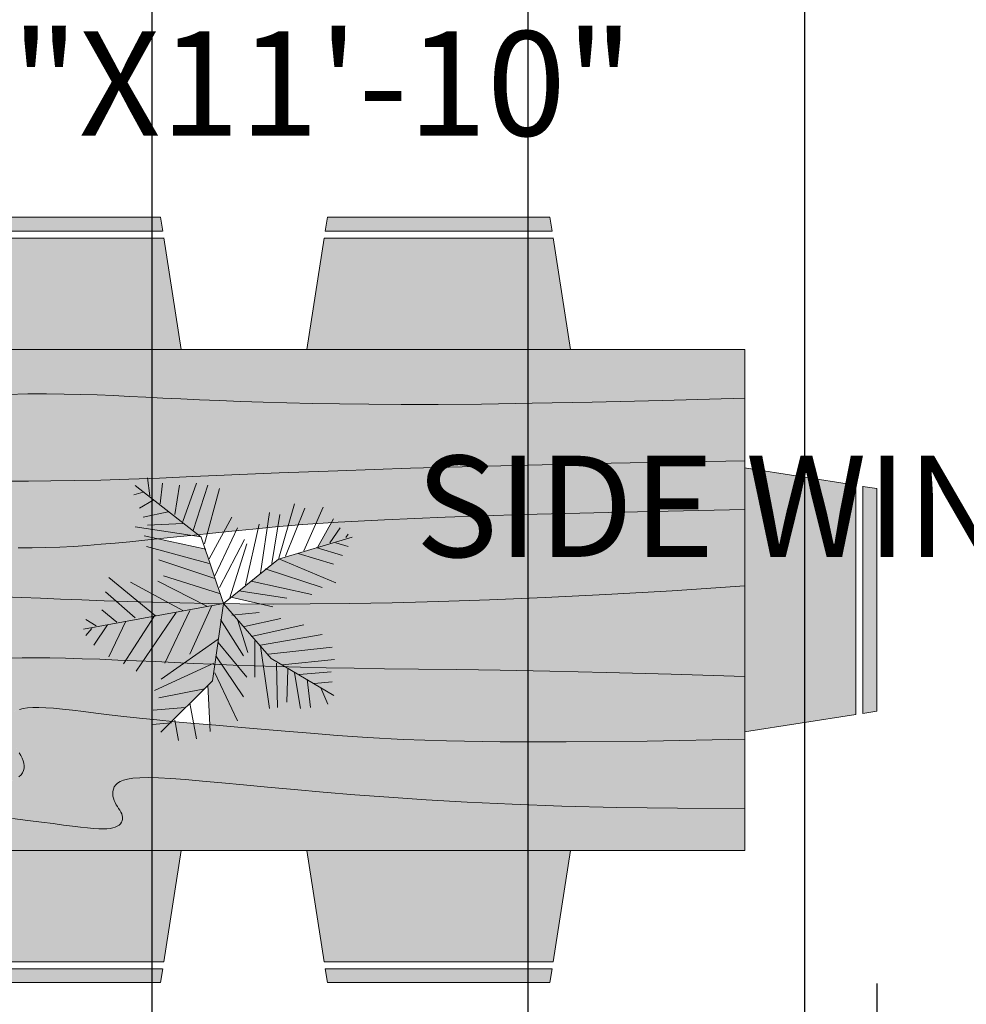
# Model space of a CAD drawing. Units: inches. Extents: x 2974 to 3443, y 2405 to 2963.
# Tile 8 of 13: x 3276 to 3341, y 2643 to 2711. Entities that reach past the tile are written whole.
import ezdxf

# ---------------------------------------------------------------- set-up
doc = ezdxf.new("R2010")
doc.units = ezdxf.units.IN
doc.header["$MEASUREMENT"] = 0
doc.layers.get('0').update_dxf_attribs({"color": 251})
for name, color, linetype, lineweight in [('A-ANNO-DIMS', 2, 'Continuous', 18), ('A-AREA-IDEN', 250, 'Continuous', 25), ('furniture', 32, 'Continuous', 18), ('greenary', 106, 'Continuous', 13)]:
    doc.layers.add(name, color=color, linetype=linetype, lineweight=lineweight)
doc.layers.add('A-FURN-PATT', color=254, linetype='Continuous', lineweight=13, true_color=0xfeeab9)
doc.styles.get("Standard").update_dxf_attribs({"font": 'arial.ttf'})
doc.dimstyles.get("Standard").update_dxf_attribs({"dimtxt": 7, "dimasz": 0.18, "dimexe": 0.18, "dimexo": 0.0625, "dimgap": 0.09, "dimtad": 0, "dimtih": 1, "dimtoh": 1, "dimzin": 0, "dimdsep": 46, "dimlunit": 3, "dimtxsty": 'Standard', "dimcen": 0.09, "dimadec": 0, "dimazin": 0, "dimtfac": 1, "dimtofl": 0, "dimtmove": 0, "dimatfit": 3, "dimfxl": 1, "dimtolj": 1, "dimtzin": 0, "dimarcsym": 0})

# ---------------------------------------------------------------- blocks, each defined once
blk = doc.blocks.new('Dining Set - 36 x 72 in.')
for p, q in [((-22, 27.5), (-22.1562, 26.50042)), ((-22, 27.5), (-6, 27.5)), ((-5.8437, 26.49966), (-6, 27.5)), ((6, 27.5), (5.8438, 26.50042)), ((6, 27.5), (22, 27.5)), ((-5.8416, 26.5), (-22.1534, 26.5)), ((22.1584, 26.5), (5.8466, 26.5)), ((-22.2343, 26.00059), (-23.4847, 17.99762)), ((-22.2304, 26), (-5.7608, 26)), ((-4.5152, 17.99762), (-5.7655, 25.99926)), ((5.7657, 26.00059), (4.5153, 17.99762)), ((5.7696, 26), (22.2392, 26)), ((36, 18), (-36, 18)), ((-36, 18), (-36, -18)), ((-44.0006, 8.23428), (-35.9976, 9.48474)), ((-45.5, 8), (-44.5004, 8.15617)), ((-45.5, 8), (-45.5, -8)), ((-44.5, -8.15843), (-44.5, 8.15338)), ((-44, 8.23041), (-44, -8.23915)), ((-44.4997, -8.15631), (-45.5, -8)), ((-35.9976, -9.48476), (-43.9993, -8.2345)), ((-36, -18), (36, -18)), ((-22.2343, -26.0006), (-23.4847, -17.99762)), ((-4.5152, -17.99762), (-5.7655, -25.99928)), ((5.7657, -26.0006), (4.5153, -17.99762)), ((-22.2304, -26), (-5.7608, -26)), ((5.7696, -26), (22.2392, -26)), ((-22, -27.5), (-22.1562, -26.50044)), ((-5.8416, -26.5), (-22.1534, -26.5)), ((-5.8437, -26.49967), (-6, -27.5)), ((6, -27.5), (5.8438, -26.50044)), ((22.1584, -26.5), (5.8466, -26.5)), ((-22, -27.5), (-6, -27.5)), ((6, -27.5), (22, -27.5))]:
    blk.add_line(p, q)
for points in [[(-36, 15), (-31.1772, 14.97754), (-26.8079, 14.91406), (-22.8538, 14.81543), (-19.276, 14.6875), (-16.0362, 14.53613), (-13.0957, 14.36718), (-10.4159, 14.18652), (-7.9583, 14), (-5.6904, 13.81315), (-3.6035, 13.63021), (-1.6954, 13.45508), (0.0365, 13.29166), (1.5945, 13.14388), (2.9811, 13.01562), (4.1988, 12.9108), (5.25, 12.83333), (6.1393, 12.78613), (6.8802, 12.76823), (7.4883, 12.77767), (7.9792, 12.8125), (8.3685, 12.87077), (8.6719, 12.95052), (8.9049, 13.0498), (9.0833, 13.16666), (9.2205, 13.29899), (9.3216, 13.44401), (9.3895, 13.59879), (9.4271, 13.76041), (9.4373, 13.92594), (9.4232, 14.09245), (9.3875, 14.257), (9.3333, 14.41666), (9.2638, 14.56917), (9.1836, 14.71484), (9.0975, 14.85465), (9.0104, 14.98958), (8.9272, 15.1206), (8.8529, 15.2487), (8.7922, 15.37483), (8.75, 15.5), (8.7305, 15.62467), (8.7344, 15.74739), (8.7617, 15.86621), (8.8125, 15.97916), (8.8867, 16.08431), (8.9844, 16.17968), (9.1055, 16.26334), (9.25, 16.33333), (9.4189, 16.38802), (9.6172, 16.42708), (9.8506, 16.45052), (10.125, 16.45833), (10.4463, 16.45052), (10.8203, 16.42708), (11.2529, 16.38802), (11.75, 16.33333), (12.3184, 16.26318), (12.9694, 16.17838), (13.7151, 16.07991), (14.5677, 15.96875), (15.5395, 15.84586), (16.6426, 15.71224)], [(-36, 10), (-28.9766, 10.14274), (-23.1725, 10.20442), (-18.4241, 10.19775), (-14.5677, 10.13541), (-11.4399, 10.03011), (-8.877, 9.89453), (-6.7154, 9.74137), (-4.7917, 9.58333), (-2.9698, 9.43082), (-1.2246, 9.28515), (0.4415, 9.14534), (2.026, 9.01041), (3.5266, 8.87939), (4.9408, 8.7513), (6.266, 8.62516), (7.5, 8.5), (8.6411, 8.37549), (9.6914, 8.2539), (10.6538, 8.13818), (11.5312, 8.03125), (12.3267, 7.93603), (13.043, 7.85547), (13.6831, 7.79248), (14.25, 7.75), (14.7471, 7.7303), (15.1797, 7.73307), (15.5537, 7.75732), (15.875, 7.80208), (16.1494, 7.86637)], [(16.1667, 11), (16.05, 11.18733), (15.9518, 11.3737), (15.8752, 11.5581), (15.8229, 11.73958), (15.798, 11.91715), (15.8034, 12.08984), (15.842, 12.25667), (15.9167, 12.41666), (16.0295, 12.56836), (16.1784, 12.70833)], [(-36, 5.5), (-30.7157, 5.3348), (-26.069, 5.20963), (-21.9946, 5.11767), (-18.4271, 5.05208), (-15.3009, 5.00602), (-12.5508, 4.97265), (-10.1112, 4.94515), (-7.9167, 4.91666), (-5.909, 4.88167), (-4.0586, 4.83984), (-2.3429, 4.79215), (-0.7396, 4.73958), (0.7739, 4.6831), (2.22, 4.6237), (3.6213, 4.56233), (5, 4.5), (6.373, 4.43782), (7.7344, 4.3776), (9.0723, 4.32129), (10.375, 4.27083), (11.6309, 4.22819), (12.8281, 4.19531), (13.9551, 4.17415), (15, 4.16666), (15.954, 4.17448), (16.819, 4.19791)], [(-36, -1), (-30.7915, -0.6591), (-26.0195, -0.38216), (-21.6519, -0.16284), (-17.6563, 0.00521), (-14.0005, 0.12833), (-10.6523, 0.21289), (-7.5796, 0.26522), (-4.75, 0.29166), (-2.134, 0.29793), (0.2878, 0.28711), (2.5317, 0.26163), (4.6146, 0.22396), (6.5529, 0.17651), (8.3633, 0.12174), (10.0623, 0.06209), (11.6667, 0), (13.1899, -0.06201), (14.6341, -0.1211), (15.9982, -0.17432), (17.2813, -0.21875)], [(-36, -6.5), (-27.1843, -6.31267), (-20.084, -6.1263), (-14.469, -5.9419), (-10.1094, -5.76042), (-6.7752, -5.58285), (-4.2363, -5.41016), (-2.2629, -5.24333), (-0.625, -5.08334), (0.8708, -4.93099), (2.2715, -4.78646), (3.5872, -4.64974), (4.8281, -4.52084), (6.0046, -4.39974), (7.127, -4.28646), (8.2053, -4.18099), (9.25, -4.08334), (10.2705, -3.99382), (11.2734, -3.91407), (12.2647, -3.84603), (13.25, -3.79167), (14.2354, -3.75293), (15.2266, -3.73177), (16.2295, -3.73015)], [(-36, -10), (-26.4022, -9.81299), (-18.4675, -9.62891), (-11.9839, -9.45069), (-6.7396, -9.28125), (-2.5226, -9.12354), (0.8789, -8.98047), (3.6769, -8.85498), (6.0833, -8.75), (8.2767, -8.66765), (10.3021, -8.60677), (12.1712, -8.56543), (13.8958, -8.54167), (15.4876, -8.53353), (16.9583, -8.53907)], [(-36, -14.5), (-30.0881, -14.33513), (-25.0332, -14.21224), (-20.7312, -14.12647), (-17.0781, -14.07292), (-13.97, -14.04671), (-11.3027, -14.04297), (-8.9724, -14.05681), (-6.875, -14.08334), (-4.9224, -14.11833), (-3.0905, -14.16016), (-1.3709, -14.20785), (0.2448, -14.26042), (1.7647, -14.3169), (3.1973, -14.3763), (4.5507, -14.43767), (5.8333, -14.5), (7.0554, -14.5621), (8.235, -14.62175), (9.3922, -14.67652), (10.5469, -14.72396), (11.7192, -14.76164), (12.929, -14.78711), (14.1965, -14.79794), (15.5417, -14.79167), (16.9933, -14.76424)]]:
    blk.add_lwpolyline(points)
blk = doc.blocks.new('dining area')
at = {"layer": 'furniture', "xscale": 0.6659924291999282, "yscale": 0.6659924291999282, "zscale": 0.6659924291999282, "rotation": 90}
blk.add_blockref('Dining Set - 36 x 72 in.', (-0.439, 20.507), dxfattribs=at)
blk = doc.blocks.new('*U13')
for p, q in [((0, 0), (-10.5, 57)), ((-8.737, 47.138), (-17.069, 52.711)), ((-10.186, 53.64), (-13.084, 55.962)), ((-9.099, 51.782), (-6.563, 55.962)), ((-7.65, 43.423), (-2.578, 49.46)), ((-7.288, 39.707), (-21.778, 46.673)), ((-5.839, 35.992), (4.667, 48.067)), ((-5.114, 27.632), (10.463, 46.673)), ((-5.114, 28.097), (-24.676, 40.636)), ((-2.941, 16.486), (8.652, 37.85)), ((44.153, 36.456), (45.239, 32.741)), ((-3.665, 19.273), (-27.574, 35.527)), ((22.055, 7.198), (27.489, 32.277)), ((27, 9), (48, 36)), ((27.127, 9.056), (31.112, 35.992)), ((35.096, 32.741), (37.27, 22.524)), ((38.719, 34.134), (41.979, 28.561)), ((-48.585, 21.131), (-49.309, 29.026)), ((-43.513, 28.561), (-42.427, 15.558)), ((-35.544, 28.097), (-24.314, 3.947)), ((16.259, 5.805), (23.142, 31.348)), ((31.836, 30.883), (32.561, 16.486)), ((43.791, 29.954), (51.036, 30.883)), ((-31.5, 4.5), (-52.5, 25.5)), ((-38.442, 26.239), (-34.819, 7.663)), ((-14.533, 2.09), (-30.834, 25.31)), ((-1.129, 6.734), (9.014, 26.704)), ((3.942, 1.625), (11.187, 24.381)), ((10.101, 3.483), (17.708, 26.239)), ((40.53, 25.775), (48.862, 24.846)), ((-24.314, 23.917), (-2.941, 13.7)), ((-47.498, 19.737), (-55.83, 18.344)), ((33.285, 16.486), (48.862, 10.913)), ((36.183, 19.737), (48.137, 17.88)), ((-40.615, 13.7), (-55.105, 10.913)), ((-20.691, 13.7), (-1.129, 4.876)), ((29.662, 12.307), (48.137, 6.269)), ((0, 0), (27, 9)), ((-33.37, 6.269), (-52.207, 5.34)), ((0, 0), (-31.5, 4.5)), ((18.07, 5.805), (35.096, -3.483)), ((24.229, 7.663), (46.688, 1.625)), ((-28.299, 3.483), (-47.86, -5.805)), ((-21.416, 3.018), (-38.079, -8.128)), ((-15.982, 2.09), (-30.11, -9.521)), ((0, 0), (-22.5, -19.5)), ((-6.563, 1.161), (-21.416, -8.128)), ((0, 0), (18, -22.5)), ((6.478, 1.625), (26.04, -8.592)), ((11.187, 3.483), (30.749, -5.805)), ((-4.752, -3.483), (-3.665, -14.629)), ((2.493, -3.019), (-1.491, -20.202)), ((1.769, -2.555), (24.229, -9.521)), ((-6.563, -5.805), (-19.967, -9.985)), ((5.029, -6.27), (2.131, -25.775)), ((-13.446, -11.378), (-8.737, -32.741)), ((-9.461, -8.592), (-6.201, -23.453)), ((9.014, -11.378), (3.58, -35.992)), ((7.565, -9.056), (32.198, -14.629)), ((-17.431, -15.094), (-42.789, -18.809)), ((-15.257, -12.772), (-30.11, -12.772)), ((-17.069, -15.094), (-12.721, -40.172)), ((12.274, -15.094), (36.907, -18.809)), ((-22.5, -19.5), (-37.5, -45)), ((-20.691, -18.345), (-17.793, -44.352)), ((14.085, -16.951), (6.478, -40.172)), ((16.259, -19.738), (36.183, -22.989)), ((-24.314, -21.596), (-42.427, -22.06)), ((-25.038, -23.918), (-22.865, -45.281)), ((18.07, -22.524), (8.289, -45.745)), ((18, -22.5), (27, -52.5)), ((18.433, -22.524), (40.53, -29.026)), ((-26.849, -26.24), (-40.253, -25.775)), ((19.157, -25.311), (38.719, -33.206)), ((-28.299, -29.026), (-42.789, -31.348)), ((-29.023, -30.884), (-27.936, -43.887)), ((20.244, -30.419), (15.897, -44.816)), ((-30.834, -34.135), (-42.427, -35.528)), ((21.331, -32.741), (39.081, -40.636)), ((-34.457, -39.708), (-40.978, -42.494)), ((-32.646, -36.921), (-31.921, -44.352)), ((22.78, -37.85), (19.519, -48.532)), ((22.78, -38.314), (34.372, -44.816)), ((24.591, -43.423), (30.749, -47.603)), ((24.591, -45.745), (23.142, -50.854)), ((26.764, -49.925), (28.213, -50.854))]:
    blk.add_line(p, q)
blk = doc.blocks.new('*D31')
at = {"layer": 'A-ANNO-DIMS', "color": 0, "lineweight": -2, "transparency": 16777216}
for p, q in [((3375.263, 2710.653), (3365.052, 2710.653)), ((3365.232, 2710.473), (3365.232, 2680.719)), ((3365.232, 2643.541), (3365.232, 2673.295)), ((3375.263, 2643.361), (3365.052, 2643.361))]:
    blk.add_line(p, q, dxfattribs=at)
at = {"layer": 'A-ANNO-DIMS', "color": 0, "transparency": 16777216}
for points in [[(3365.202, 2710.473), (3365.262, 2710.473), (3365.232, 2710.653)], [(3365.202, 2643.541), (3365.262, 2643.541), (3365.232, 2643.361)]]:
    blk.add_solid(points, dxfattribs=at)
at = {"layer": 'Defpoints', "color": 0, "transparency": 16777216}
for p in [(3365.232, 2710.653), (3375.326, 2710.653), (3375.326, 2643.361)]:
    blk.add_point(p, dxfattribs=at)
at = {"layer": 'A-ANNO-DIMS', "color": 0, "transparency": 16777216, "insert": (3365.232, 2677.007), "char_height": 7, "attachment_point": 5}
blk.add_mtext('\\A1;SIDE WINDOW 5\'-7 1/2" TYP.', dxfattribs=at)
blk = doc.blocks.new('*D47')
at = {"layer": 'A-ANNO-DIMS', "color": 0, "lineweight": -2, "transparency": 16777216}
for p, q in [((3247.425, 2644.017), (3247.425, 2630.764)), ((3334.991, 2644.017), (3334.991, 2630.764)), ((3247.425, 2630.944), (3247.245, 2630.944)), ((3334.811, 2630.944), (3247.605, 2630.944))]:
    blk.add_line(p, q, dxfattribs=at)
at = {"layer": 'A-ANNO-DIMS', "color": 0, "transparency": 16777216}
for points in [[(3247.605, 2630.974), (3247.605, 2630.914), (3247.425, 2630.944)], [(3334.811, 2630.974), (3334.811, 2630.914), (3334.991, 2630.944)]]:
    blk.add_solid(points, dxfattribs=at)
at = {"layer": 'Defpoints', "color": 0, "transparency": 16777216}
for p in [(3247.425, 2644.079), (3334.991, 2644.079), (3247.425, 2630.944)]:
    blk.add_point(p, dxfattribs=at)
at = {"layer": 'A-ANNO-DIMS', "color": 0, "transparency": 16777216, "insert": (3200.531, 2630.944), "char_height": 7, "attachment_point": 5}
blk.add_mtext('\\A1;DINING SET 7\'-3 1/2"', dxfattribs=at)
blk = doc.blocks.new('*D62')
at = {"layer": 'A-ANNO-DIMS', "color": 0, "lineweight": -2, "transparency": 16777216}
for p, q in [((3267.326, 2609.251), (3267.326, 2952.678)), ((3267.506, 2952.498), (3281.115, 2952.498)), ((3329.823, 2952.498), (3316.214, 2952.498)), ((3330.003, 2609.251), (3330.003, 2952.678))]:
    blk.add_line(p, q, dxfattribs=at)
at = {"layer": 'A-ANNO-DIMS', "color": 0, "transparency": 16777216}
for points in [[(3267.506, 2952.528), (3267.506, 2952.468), (3267.326, 2952.498)], [(3329.823, 2952.528), (3329.823, 2952.468), (3330.003, 2952.498)]]:
    blk.add_solid(points, dxfattribs=at)
at = {"layer": 'Defpoints', "color": 0, "transparency": 16777216}
for p in [(3330.003, 2952.498), (3267.326, 2609.188), (3330.003, 2609.188)]:
    blk.add_point(p, dxfattribs=at)
at = {"layer": 'A-ANNO-DIMS', "color": 0, "transparency": 16777216, "insert": (3298.665, 2952.498), "char_height": 7, "attachment_point": 5}
blk.add_mtext('\\A1;5\'-2 1/2"', dxfattribs=at)
blk = doc.blocks.new('*D63')
at = {"layer": 'A-ANNO-DIMS', "color": 0, "lineweight": -2, "transparency": 16777216}
for p, q in [((3244.826, 2751.126), (3244.826, 2414.917)), ((3284.826, 2751.126), (3284.826, 2414.917)), ((3245.006, 2415.097), (3255.434, 2415.097)), ((3284.646, 2415.097), (3274.217, 2415.097))]:
    blk.add_line(p, q, dxfattribs=at)
at = {"layer": 'A-ANNO-DIMS', "color": 0, "transparency": 16777216}
for points in [[(3245.006, 2415.127), (3245.006, 2415.067), (3244.826, 2415.097)], [(3284.646, 2415.127), (3284.646, 2415.067), (3284.826, 2415.097)]]:
    blk.add_solid(points, dxfattribs=at)
at = {"layer": 'Defpoints', "color": 0, "transparency": 16777216}
for p in [(3244.826, 2751.188), (3284.826, 2751.188), (3284.826, 2415.097)]:
    blk.add_point(p, dxfattribs=at)
at = {"layer": 'A-ANNO-DIMS', "color": 0, "transparency": 16777216, "insert": (3264.826, 2415.097), "char_height": 7, "attachment_point": 5}
blk.add_mtext('\\A1;3\'-4"', dxfattribs=at)
blk = doc.blocks.new('*D78')
at = {"layer": 'A-ANNO-DIMS', "color": 0, "lineweight": -2, "transparency": 16777216}
for p, q in [((3267.326, 2480.251), (3267.326, 2952.678)), ((3267.506, 2952.498), (3271.548, 2952.498)), ((3310.684, 2952.498), (3306.642, 2952.498)), ((3310.864, 2481.932), (3310.864, 2952.678))]:
    blk.add_line(p, q, dxfattribs=at)
at = {"layer": 'A-ANNO-DIMS', "color": 0, "transparency": 16777216}
for points in [[(3267.506, 2952.528), (3267.506, 2952.468), (3267.326, 2952.498)], [(3310.684, 2952.528), (3310.684, 2952.468), (3310.864, 2952.498)]]:
    blk.add_solid(points, dxfattribs=at)
at = {"layer": 'Defpoints', "color": 0, "transparency": 16777216}
for p in [(3310.864, 2952.498), (3310.864, 2481.869), (3267.326, 2480.188)]:
    blk.add_point(p, dxfattribs=at)
at = {"layer": 'A-ANNO-DIMS', "color": 0, "transparency": 16777216, "insert": (3289.095, 2952.498), "char_height": 7, "attachment_point": 5}
blk.add_mtext('\\A1;3\'-7 1/2"', dxfattribs=at)

msp = doc.modelspace()

# ---------------------------------------------------------------- hatches: boundary and pattern name
at = {"layer": 'A-FURN-PATT'}
h = msp.add_hatch(color=256, dxfattribs=at)
h.dxf.hatch_style = 1
h.paths.add_polyline_path([(3285.66, 2695.56), (3269.813, 2695.56), (3268.61, 2687.862), (3286.863, 2687.862)])
h.paths.add_polyline_path([(3285.434, 2697.003), (3270.038, 2697.003), (3269.888, 2696.041), (3285.585, 2696.041)])
h.paths.add_polyline_path([(3312.603, 2695.56), (3296.756, 2695.56), (3295.553, 2687.862), (3313.806, 2687.862)])
h.paths.add_polyline_path([(3312.378, 2697.003), (3296.981, 2697.003), (3296.831, 2696.041), (3312.528, 2696.041)])
h.paths.add_polyline_path([(3256.566, 2679.668), (3248.868, 2678.465), (3248.868, 2662.618), (3256.566, 2661.415)])
h.paths.add_polyline_path([(3248.387, 2678.39), (3247.425, 2678.239), (3247.425, 2662.843), (3248.387, 2662.693)])
h.paths.add_polyline_path([(3286.863, 2653.221), (3268.61, 2653.221), (3269.813, 2645.522), (3285.66, 2645.522)])
h.paths.add_polyline_path([(3285.585, 2645.041), (3269.888, 2645.041), (3270.038, 2644.079), (3285.434, 2644.079)])
h.paths.add_polyline_path([(3312.528, 2645.041), (3296.831, 2645.041), (3296.981, 2644.079), (3312.378, 2644.079)])
h.paths.add_polyline_path([(3313.806, 2653.221), (3295.553, 2653.221), (3296.756, 2645.522), (3312.603, 2645.522)])
h.paths.add_polyline_path([(3333.547, 2678.465), (3325.849, 2679.668), (3325.849, 2661.415), (3333.547, 2662.618)])
h.paths.add_polyline_path([(3334.991, 2678.239), (3334.028, 2678.39), (3334.028, 2662.693), (3334.991, 2662.843)])
h = msp.add_hatch(color=256, dxfattribs=at)
h.dxf.hatch_style = 1
h.paths.add_polyline_path([(3325.849, 2687.862), (3256.566, 2687.862), (3256.566, 2683.051), (3260.581, 2683.537), (3264.012, 2683.923), (3266.929, 2684.22), (3269.402, 2684.439), (3271.5, 2684.592), (3273.295, 2684.691), (3274.856, 2684.748), (3276.253, 2684.775), (3277.547, 2684.781), (3278.767, 2684.77), (3279.931, 2684.746), (3281.059, 2684.71), (3282.17, 2684.664), (3283.284, 2684.611), (3284.419, 2684.554), (3285.595, 2684.494), (3286.829, 2684.434), (3288.131, 2684.375), (3289.51, 2684.318), (3290.972, 2684.263), (3292.527, 2684.213), (3294.182, 2684.167), (3295.944, 2684.127), (3297.823, 2684.093), (3299.842, 2684.068), (3302.084, 2684.054), (3304.651, 2684.058), (3307.641, 2684.083), (3311.157, 2684.135), (3315.296, 2684.217), (3320.16, 2684.335), (3325.849, 2684.494)])
h.paths.add_polyline_path([(3325.849, 2684.494), (3320.16, 2684.335), (3315.296, 2684.217), (3311.157, 2684.135), (3307.641, 2684.083), (3304.651, 2684.058), (3302.084, 2684.054), (3299.842, 2684.068), (3297.823, 2684.093), (3295.944, 2684.127), (3294.182, 2684.167), (3292.527, 2684.213), (3290.972, 2684.263), (3289.51, 2684.318), (3288.131, 2684.375), (3286.829, 2684.434), (3285.595, 2684.494), (3284.419, 2684.554), (3283.284, 2684.611), (3282.17, 2684.664), (3281.059, 2684.71), (3279.931, 2684.746), (3278.767, 2684.77), (3277.547, 2684.781), (3276.253, 2684.775), (3274.856, 2684.748), (3273.295, 2684.691), (3271.5, 2684.592), (3269.402, 2684.439), (3266.929, 2684.22), (3264.012, 2683.923), (3260.581, 2683.537), (3256.566, 2683.051), (3256.566, 2679.683), (3257.49, 2679.672), (3258.448, 2679.642), (3259.434, 2679.596), (3260.436, 2679.537), (3261.445, 2679.469), (3262.453, 2679.395), (3263.449, 2679.318), (3264.425, 2679.242), (3265.375, 2679.168), (3266.308, 2679.099), (3267.24, 2679.035), (3268.184, 2678.976), (3269.154, 2678.923), (3270.165, 2678.875), (3271.23, 2678.834), (3272.364, 2678.801), (3273.58, 2678.775), (3274.89, 2678.758), (3276.305, 2678.753), (3277.836, 2678.761), (3279.496, 2678.783), (3281.295, 2678.823), (3283.244, 2678.882), (3285.354, 2678.961), (3287.67, 2679.062), (3290.362, 2679.183), (3293.635, 2679.32), (3297.693, 2679.472), (3302.739, 2679.635), (3308.978, 2679.807), (3316.614, 2679.984), (3325.849, 2680.164)])
h.paths.add_polyline_path([(3284.707, 2677.646), (3284.542, 2678.931), (3283.244, 2678.882), (3281.295, 2678.823), (3279.496, 2678.783), (3277.836, 2678.761), (3276.305, 2678.753), (3274.89, 2678.758), (3273.58, 2678.775), (3272.364, 2678.801), (3271.23, 2678.834), (3270.165, 2678.875), (3269.154, 2678.923), (3268.184, 2678.976), (3267.24, 2679.035), (3266.308, 2679.099), (3265.375, 2679.168), (3264.425, 2679.242), (3263.449, 2679.318), (3262.453, 2679.395), (3261.445, 2679.469), (3260.436, 2679.537), (3259.434, 2679.596), (3258.448, 2679.642), (3257.49, 2679.672), (3256.656, 2679.682), (3256.566, 2679.668), (3256.566, 2675.834), (3257.118, 2675.982), (3257.69, 2676.07), (3258.277, 2676.106), (3258.877, 2676.099), (3259.486, 2676.056), (3260.102, 2675.986), (3260.72, 2675.896), (3261.338, 2675.794), (3261.954, 2675.687), (3262.574, 2675.576), (3263.206, 2675.463), (3263.859, 2675.348), (3264.539, 2675.23), (3265.256, 2675.111), (3266.017, 2674.992), (3266.831, 2674.871), (3267.701, 2674.752), (3268.621, 2674.635), (3269.581, 2674.523), (3270.569, 2674.42), (3271.577, 2674.329), (3272.593, 2674.251), (3273.607, 2674.191), (3274.609, 2674.15), (3275.591, 2674.131), (3276.556, 2674.132), (3277.51, 2674.153), (3278.458, 2674.19), (3279.406, 2674.242), (3280.36, 2674.308), (3281.325, 2674.384), (3282.307, 2674.47), (3283.312, 2674.564), (3284.35, 2674.666), (3285.43, 2674.775), (3286.562, 2674.891), (3287.756, 2675.015), (3288.049, 2675.046)])
h.paths.add_polyline_path([(3288.532, 2674.053), (3285.273, 2674.759), (3284.35, 2674.666), (3283.312, 2674.564), (3282.307, 2674.47), (3281.325, 2674.384), (3280.36, 2674.308), (3279.406, 2674.242), (3278.458, 2674.19), (3277.51, 2674.153), (3276.556, 2674.132), (3275.591, 2674.131), (3274.609, 2674.15), (3273.607, 2674.191), (3272.593, 2674.251), (3271.577, 2674.329), (3270.569, 2674.42), (3269.581, 2674.523), (3268.621, 2674.635), (3267.701, 2674.752), (3266.831, 2674.871), (3266.017, 2674.992), (3265.256, 2675.111), (3264.539, 2675.23), (3263.859, 2675.348), (3263.206, 2675.463), (3262.574, 2675.576), (3261.954, 2675.687), (3261.338, 2675.794), (3260.72, 2675.896), (3260.102, 2675.986), (3259.486, 2676.056), (3258.877, 2676.099), (3258.277, 2676.106), (3257.69, 2676.07), (3257.118, 2675.982), (3256.566, 2675.834), (3256.566, 2670.541), (3256.88, 2670.541), (3257.044, 2670.502), (3257.158, 2670.474), (3257.327, 2670.434), (3257.569, 2670.381), (3257.899, 2670.314), (3258.307, 2670.237), (3258.779, 2670.154), (3259.298, 2670.07), (3259.849, 2669.99), (3260.416, 2669.919), (3260.984, 2669.86), (3261.538, 2669.82), (3262.065, 2669.8), (3262.568, 2669.802), (3263.052, 2669.822), (3263.523, 2669.86), (3263.986, 2669.912), (3264.447, 2669.977), (3264.913, 2670.054), (3265.387, 2670.14), (3265.877, 2670.234), (3266.391, 2670.331), (3266.936, 2670.428), (3267.522, 2670.521), (3268.157, 2670.607), (3268.849, 2670.682), (3269.607, 2670.741), (3270.439, 2670.782), (3271.352, 2670.801), (3272.347, 2670.801), (3273.423, 2670.783), (3274.579, 2670.752), (3275.813, 2670.709), (3277.126, 2670.658), (3278.516, 2670.601), (3279.981, 2670.541), (3281.525, 2670.481), (3283.16, 2670.424), (3284.902, 2670.371), (3286.767, 2670.326), (3288.772, 2670.289), (3289.667, 2670.279), (3289.783, 2670.301)], flags=16)
h.paths.add_polyline_path([(3325.849, 2680.164), (3316.614, 2679.984), (3308.978, 2679.807), (3302.739, 2679.635), (3297.693, 2679.472), (3293.635, 2679.32), (3290.362, 2679.183), (3287.67, 2679.062), (3285.354, 2678.961), (3284.542, 2678.931), (3284.707, 2677.646), (3288.049, 2675.046), (3289.022, 2675.147), (3290.37, 2675.286), (3291.809, 2675.433), (3293.55, 2675.603), (3293.55, 2675.601), (3295.284, 2675.747), (3297.727, 2675.913), (3300.936, 2676.084), (3305.131, 2676.259), (3310.534, 2676.436), (3317.366, 2676.616), (3325.849, 2676.796)])
h.paths.add_polyline_path([(3325.849, 2676.796), (3317.366, 2676.616), (3310.534, 2676.436), (3305.131, 2676.259), (3300.936, 2676.084), (3297.727, 2675.913), (3297.25, 2675.881), (3296.279, 2674.149), (3296.261, 2674.155), (3293.605, 2673.358), (3290.309, 2670.721), (3292.302, 2670.259), (3293.261, 2670.255), (3295.779, 2670.261), (3298.501, 2670.286), (3301.458, 2670.336), (3304.68, 2670.418), (3308.198, 2670.536), (3312.043, 2670.698), (3316.245, 2670.909), (3320.837, 2671.175), (3325.849, 2671.503)])
h.paths.add_polyline_path([(3325.849, 2671.503), (3320.837, 2671.175), (3316.245, 2670.909), (3312.043, 2670.698), (3308.198, 2670.536), (3304.68, 2670.418), (3301.458, 2670.336), (3298.501, 2670.286), (3295.779, 2670.261), (3293.261, 2670.255), (3290.931, 2670.265), (3289.803, 2670.278), (3292.302, 2667.394), (3292.338, 2667.4), (3292.346, 2667.343), (3293.095, 2666.479), (3294.056, 2665.913), (3295.113, 2665.884), (3296.894, 2665.844), (3298.826, 2665.81), (3300.937, 2665.783), (3303.285, 2665.756), (3305.931, 2665.724), (3308.94, 2665.68), (3312.372, 2665.617), (3316.293, 2665.528), (3320.764, 2665.408), (3325.849, 2665.249)])
h.paths.add_polyline_path([(3325.849, 2665.249), (3320.764, 2665.408), (3316.293, 2665.528), (3312.372, 2665.617), (3308.94, 2665.68), (3305.931, 2665.724), (3303.285, 2665.756), (3300.937, 2665.783), (3298.826, 2665.81), (3296.894, 2665.844), (3295.113, 2665.884), (3294.056, 2665.913), (3293.095, 2666.479), (3292.346, 2667.343), (3289.803, 2670.278), (3289.78, 2670.278), (3289.019, 2664.95), (3288.717, 2664.649), (3288.853, 2661.906), (3289.258, 2661.871), (3290.783, 2661.741), (3292.386, 2661.607), (3294.066, 2661.466), (3295.819, 2661.32), (3297.67, 2661.168), (3299.75, 2661.02), (3302.216, 2660.89), (3305.226, 2660.788), (3308.937, 2660.728), (3313.506, 2660.722), (3319.091, 2660.781), (3325.849, 2660.919)])
h.paths.add_polyline_path([(3289.431, 2667.834), (3289.783, 2670.301), (3288.532, 2674.053), (3285.273, 2674.759), (3284.35, 2674.666), (3283.312, 2674.564), (3282.307, 2674.47), (3281.325, 2674.384), (3280.36, 2674.308), (3279.406, 2674.242), (3278.458, 2674.19), (3277.51, 2674.153), (3276.556, 2674.132), (3275.591, 2674.131), (3274.609, 2674.15), (3273.607, 2674.191), (3272.593, 2674.251), (3271.577, 2674.329), (3270.569, 2674.42), (3269.581, 2674.523), (3268.621, 2674.635), (3267.701, 2674.752), (3266.831, 2674.871), (3266.017, 2674.992), (3265.256, 2675.111), (3264.539, 2675.23), (3263.859, 2675.348), (3263.206, 2675.463), (3262.574, 2675.576), (3261.954, 2675.687), (3261.338, 2675.794), (3260.72, 2675.896), (3260.102, 2675.986), (3259.486, 2676.056), (3258.877, 2676.099), (3258.277, 2676.106), (3257.69, 2676.07), (3257.118, 2675.982), (3256.566, 2675.834), (3256.566, 2670.541), (3256.88, 2670.541), (3257.044, 2670.502), (3257.158, 2670.474), (3257.442, 2670.406), (3257.569, 2670.381), (3257.258, 2670.449), (3257.044, 2670.502), (3256.88, 2670.541), (3256.566, 2670.541), (3256.566, 2666.211), (3258.06, 2665.872), (3259.317, 2665.575), (3260.368, 2665.315), (3261.247, 2665.088), (3261.988, 2664.892), (3262.622, 2664.723), (3263.183, 2664.575), (3263.703, 2664.447), (3264.21, 2664.334), (3264.707, 2664.238), (3265.19, 2664.158), (3265.658, 2664.096), (3266.107, 2664.053), (3266.534, 2664.03), (3266.936, 2664.027), (3267.312, 2664.046), (3267.658, 2664.087), (3267.977, 2664.149), (3268.272, 2664.229), (3268.545, 2664.327), (3268.799, 2664.439), (3269.037, 2664.565), (3269.262, 2664.702), (3269.477, 2664.848), (3269.685, 2665.002), (3270.053, 2665.282), (3270.339, 2665.479), (3270.592, 2665.635), (3270.875, 2665.784), (3271.196, 2665.923), (3271.562, 2666.051), (3271.98, 2666.163), (3272.455, 2666.261), (3272.992, 2666.344), (3273.596, 2666.412), (3274.272, 2666.464), (3275.024, 2666.502), (3275.856, 2666.524), (3276.774, 2666.532), (3277.779, 2666.525), (3278.864, 2666.504), (3280.016, 2666.473), (3281.224, 2666.432), (3282.478, 2666.383), (3283.765, 2666.329), (3285.075, 2666.271), (3286.397, 2666.211), (3287.075, 2666.18)])
h.paths.add_polyline_path([(3289.019, 2664.95), (3289.431, 2667.834), (3287.075, 2666.18), (3286.397, 2666.211), (3285.075, 2666.271), (3283.765, 2666.329), (3282.478, 2666.383), (3281.224, 2666.432), (3280.016, 2666.473), (3278.864, 2666.504), (3277.779, 2666.525), (3276.774, 2666.532), (3275.856, 2666.524), (3275.024, 2666.502), (3274.272, 2666.464), (3273.596, 2666.412), (3272.992, 2666.344), (3272.455, 2666.261), (3271.98, 2666.163), (3271.562, 2666.051), (3271.196, 2665.923), (3270.875, 2665.784), (3270.592, 2665.635), (3270.339, 2665.479), (3270.053, 2665.282), (3269.536, 2664.889), (3269.144, 2664.621), (3268.799, 2664.439), (3268.545, 2664.327), (3268.272, 2664.229), (3267.977, 2664.149), (3267.658, 2664.087), (3267.312, 2664.046), (3266.936, 2664.027), (3266.534, 2664.03), (3266.107, 2664.053), (3265.658, 2664.096), (3265.19, 2664.158), (3264.707, 2664.238), (3264.21, 2664.334), (3263.703, 2664.447), (3263.183, 2664.575), (3262.622, 2664.723), (3261.988, 2664.892), (3261.247, 2665.088), (3260.368, 2665.315), (3259.317, 2665.575), (3258.06, 2665.872), (3256.566, 2666.211), (3256.566, 2661.881), (3259.267, 2661.372), (3261.616, 2660.924), (3263.647, 2660.53), (3265.392, 2660.182), (3266.883, 2659.873), (3268.153, 2659.597), (3269.234, 2659.347), (3270.158, 2659.114), (3270.956, 2658.895), (3271.643, 2658.69), (3272.233, 2658.503), (3272.739, 2658.338), (3273.177, 2658.196), (3273.558, 2658.083), (3273.897, 2658), (3274.208, 2657.952), (3274.501, 2657.94), (3274.776, 2657.962), (3275.03, 2658.014), (3275.26, 2658.092), (3275.465, 2658.193), (3275.64, 2658.313), (3275.783, 2658.447), (3275.892, 2658.593), (3275.964, 2658.747), (3276.001, 2658.908), (3276.006, 2659.074), (3275.982, 2659.245), (3275.932, 2659.419), (3275.858, 2659.597), (3275.764, 2659.776), (3275.651, 2659.956), (3275.524, 2660.137), (3275.388, 2660.317), (3275.135, 2660.643), (3274.902, 2660.965), (3274.71, 2661.317), (3274.621, 2661.669), (3274.646, 2662.019), (3274.778, 2662.344), (3275.01, 2662.628), (3275.338, 2662.855), (3275.668, 2662.972), (3275.932, 2663.034), (3276.241, 2663.077), (3276.601, 2663.1), (3277.017, 2663.103), (3277.496, 2663.084), (3278.041, 2663.043), (3278.657, 2662.982), (3279.346, 2662.905), (3280.112, 2662.813), (3280.956, 2662.71), (3281.882, 2662.599), (3282.893, 2662.482), (3283.991, 2662.362), (3285.178, 2662.242), (3286.212, 2662.143)])
h.paths.add_polyline_path([(3288.532, 2674.053), (3285.273, 2674.759), (3284.35, 2674.666), (3283.312, 2674.564), (3282.307, 2674.47), (3281.325, 2674.384), (3280.36, 2674.308), (3279.406, 2674.242), (3278.458, 2674.19), (3277.51, 2674.153), (3276.556, 2674.132), (3275.591, 2674.131), (3274.609, 2674.15), (3273.607, 2674.191), (3272.593, 2674.251), (3271.577, 2674.329), (3270.569, 2674.42), (3269.581, 2674.523), (3268.621, 2674.635), (3267.701, 2674.752), (3266.831, 2674.871), (3266.017, 2674.992), (3265.256, 2675.111), (3264.539, 2675.23), (3263.859, 2675.348), (3263.206, 2675.463), (3262.574, 2675.576), (3261.954, 2675.687), (3261.338, 2675.794), (3260.72, 2675.896), (3260.102, 2675.986), (3259.486, 2676.056), (3258.877, 2676.099), (3258.277, 2676.106), (3257.69, 2676.07), (3257.118, 2675.982), (3256.566, 2675.834), (3256.566, 2670.541), (3256.716, 2670.541), (3256.88, 2670.541), (3257.044, 2670.502), (3257.158, 2670.474), (3257.327, 2670.434), (3257.569, 2670.381), (3257.899, 2670.314), (3258.307, 2670.237), (3258.779, 2670.154), (3259.298, 2670.07), (3259.849, 2669.99), (3260.416, 2669.919), (3260.984, 2669.86), (3261.538, 2669.82), (3262.065, 2669.8), (3262.568, 2669.802), (3263.052, 2669.822), (3263.523, 2669.86), (3263.986, 2669.912), (3264.447, 2669.977), (3264.913, 2670.054), (3265.387, 2670.14), (3265.877, 2670.234), (3266.391, 2670.331), (3266.936, 2670.428), (3267.522, 2670.521), (3268.157, 2670.607), (3268.849, 2670.682), (3269.607, 2670.741), (3270.439, 2670.782), (3271.352, 2670.801), (3272.347, 2670.801), (3273.423, 2670.783), (3274.579, 2670.752), (3275.813, 2670.709), (3277.126, 2670.658), (3278.516, 2670.601), (3279.981, 2670.541), (3281.525, 2670.481), (3283.16, 2670.424), (3284.902, 2670.371), (3286.767, 2670.326), (3288.772, 2670.289), (3289.667, 2670.279), (3289.783, 2670.301)], flags=17)
h.paths.add_polyline_path([(3275.26, 2658.092), (3275.465, 2658.193), (3275.64, 2658.313), (3275.783, 2658.447), (3275.892, 2658.593), (3275.964, 2658.747), (3276.001, 2658.908), (3276.006, 2659.074), (3275.982, 2659.245), (3275.932, 2659.419), (3275.858, 2659.597), (3275.764, 2659.776), (3275.651, 2659.956), (3275.524, 2660.137), (3275.388, 2660.317), (3275.038, 2660.768), (3274.979, 2660.858), (3274.902, 2660.965), (3274.71, 2661.317), (3274.621, 2661.669), (3274.646, 2662.019), (3274.778, 2662.344), (3275.01, 2662.628), (3275.338, 2662.855), (3275.668, 2662.972), (3275.932, 2663.034), (3276.241, 2663.077), (3276.601, 2663.1), (3277.017, 2663.103), (3277.496, 2663.084), (3278.041, 2663.043), (3278.657, 2662.982), (3279.346, 2662.905), (3280.112, 2662.813), (3280.956, 2662.71), (3281.882, 2662.599), (3282.893, 2662.482), (3283.991, 2662.362), (3285.178, 2662.242), (3286.212, 2662.143), (3289.019, 2664.95), (3289.431, 2667.834), (3287.075, 2666.18), (3286.397, 2666.211), (3285.075, 2666.271), (3283.765, 2666.329), (3282.478, 2666.383), (3281.224, 2666.432), (3280.016, 2666.473), (3278.864, 2666.504), (3277.779, 2666.525), (3276.774, 2666.532), (3275.856, 2666.524), (3275.024, 2666.502), (3274.272, 2666.464), (3273.596, 2666.412), (3272.992, 2666.344), (3272.455, 2666.261), (3271.98, 2666.163), (3271.562, 2666.051), (3271.196, 2665.923), (3270.875, 2665.784), (3270.592, 2665.635), (3270.339, 2665.479), (3270.053, 2665.282), (3269.536, 2664.889), (3269.144, 2664.621), (3268.799, 2664.439), (3268.545, 2664.327), (3268.272, 2664.229), (3267.977, 2664.149), (3267.658, 2664.087), (3267.312, 2664.046), (3266.936, 2664.027), (3266.534, 2664.03), (3266.107, 2664.053), (3265.658, 2664.096), (3265.19, 2664.158), (3264.707, 2664.238), (3264.21, 2664.334), (3263.703, 2664.447), (3263.183, 2664.575), (3262.622, 2664.723), (3261.988, 2664.892), (3261.247, 2665.088), (3260.368, 2665.315), (3259.317, 2665.575), (3258.06, 2665.872), (3256.566, 2666.211), (3256.566, 2661.881), (3259.267, 2661.372), (3261.616, 2660.924), (3263.647, 2660.53), (3265.392, 2660.182), (3266.883, 2659.873), (3268.153, 2659.597), (3269.234, 2659.347), (3270.158, 2659.114), (3270.956, 2658.895), (3271.643, 2658.69), (3272.233, 2658.503), (3272.739, 2658.338), (3273.177, 2658.196), (3273.558, 2658.083), (3273.897, 2658), (3274.208, 2657.952), (3274.501, 2657.94), (3274.776, 2657.962), (3275.03, 2658.014)], flags=16)
h.paths.add_polyline_path([(3286.212, 2662.143), (3285.178, 2662.242), (3283.991, 2662.362), (3282.893, 2662.482), (3281.882, 2662.599), (3280.956, 2662.71), (3280.112, 2662.813), (3279.346, 2662.905), (3278.657, 2662.982), (3278.041, 2663.043), (3277.496, 2663.084), (3277.017, 2663.103), (3276.601, 2663.1), (3276.241, 2663.077), (3275.932, 2663.034), (3275.668, 2662.972), (3275.443, 2662.892), (3275.253, 2662.795), (3275.09, 2662.683), (3274.951, 2662.555), (3274.836, 2662.415), (3274.745, 2662.263), (3274.679, 2662.101), (3274.64, 2661.933), (3274.628, 2661.758), (3274.644, 2661.58), (3274.689, 2661.4), (3274.763, 2661.219), (3274.862, 2661.039), (3274.979, 2660.858), (3275.11, 2660.678), (3275.248, 2660.498), (3275.488, 2660.188), (3275.72, 2659.858), (3275.908, 2659.502), (3276.009, 2659.153), (3275.998, 2658.821), (3275.855, 2658.515), (3275.566, 2658.243), (3275.153, 2658.039), (3274.776, 2657.962), (3274.501, 2657.94), (3274.208, 2657.952), (3273.897, 2658), (3273.558, 2658.083), (3273.177, 2658.196), (3272.739, 2658.338), (3272.233, 2658.503), (3271.643, 2658.69), (3270.956, 2658.895), (3270.158, 2659.114), (3269.234, 2659.347), (3268.153, 2659.597), (3266.883, 2659.873), (3265.392, 2660.182), (3263.647, 2660.53), (3261.616, 2660.924), (3259.267, 2661.372), (3256.566, 2661.881), (3256.566, 2657.07), (3259.035, 2656.889), (3261.385, 2656.71), (3263.609, 2656.533), (3265.703, 2656.358), (3267.659, 2656.187), (3269.472, 2656.021), (3271.136, 2655.86), (3272.644, 2655.706), (3273.994, 2655.56), (3275.193, 2655.422), (3276.255, 2655.293), (3277.19, 2655.175), (3278.01, 2655.068), (3278.728, 2654.973), (3279.354, 2654.892), (3279.901, 2654.824), (3280.38, 2654.772), (3280.796, 2654.734), (3281.156, 2654.712), (3281.465, 2654.704), (3281.729, 2654.712), (3281.954, 2654.734), (3282.144, 2654.772), (3282.307, 2654.824), (3282.446, 2654.892), (3282.563, 2654.972), (3282.657, 2655.064), (3282.728, 2655.165), (3282.777, 2655.274), (3282.803, 2655.388), (3282.807, 2655.506), (3282.788, 2655.626), (3282.747, 2655.747), (3282.689, 2655.868), (3282.618, 2655.991), (3282.538, 2656.117), (3282.335, 2656.431), (3282.191, 2656.747), (3282.122, 2657.065), (3282.142, 2657.385), (3282.273, 2657.684), (3282.54, 2657.942), (3282.863, 2658.079), (3283.155, 2658.156), (3283.53, 2658.212), (3284.002, 2658.246), (3284.587, 2658.255), (3285.3, 2658.238), (3286.156, 2658.192), (3287.168, 2658.118), (3288.339, 2658.017), (3289.674, 2657.893), (3291.173, 2657.751), (3292.839, 2657.594), (3294.675, 2657.425), (3296.684, 2657.249), (3298.866, 2657.07), (3301.231, 2656.89), (3303.809, 2656.716), (3306.639, 2656.554), (3309.756, 2656.408), (3313.199, 2656.285), (3317.004, 2656.19), (3321.208, 2656.129), (3325.849, 2656.107), (3325.849, 2660.919), (3319.091, 2660.781), (3313.506, 2660.722), (3308.937, 2660.728), (3305.226, 2660.788), (3302.216, 2660.89), (3299.75, 2661.02), (3297.67, 2661.168), (3295.819, 2661.32), (3294.066, 2661.466), (3292.386, 2661.607), (3290.783, 2661.741), (3289.258, 2661.871), (3287.725, 2662.005), (3287.725, 2662.005), (3286.211, 2662.142)])
h.paths.add_polyline_path([(3289.019, 2664.95), (3289.431, 2667.834), (3287.075, 2666.18), (3286.397, 2666.211), (3285.075, 2666.271), (3283.765, 2666.329), (3282.478, 2666.383), (3281.224, 2666.432), (3280.016, 2666.473), (3278.864, 2666.504), (3277.779, 2666.525), (3276.774, 2666.532), (3275.856, 2666.524), (3275.024, 2666.502), (3274.272, 2666.464), (3273.596, 2666.412), (3272.992, 2666.344), (3272.455, 2666.261), (3271.98, 2666.163), (3271.562, 2666.051), (3271.196, 2665.923), (3270.875, 2665.784), (3270.592, 2665.635), (3270.339, 2665.479), (3270.053, 2665.282), (3269.536, 2664.889), (3269.144, 2664.621), (3268.799, 2664.439), (3268.545, 2664.327), (3268.272, 2664.229), (3267.977, 2664.149), (3267.658, 2664.087), (3267.312, 2664.046), (3266.936, 2664.027), (3266.534, 2664.03), (3266.107, 2664.053), (3265.658, 2664.096), (3265.19, 2664.158), (3264.707, 2664.238), (3264.21, 2664.334), (3263.703, 2664.447), (3263.183, 2664.575), (3262.622, 2664.723), (3261.988, 2664.892), (3261.247, 2665.088), (3260.368, 2665.315), (3259.317, 2665.575), (3258.06, 2665.872), (3256.566, 2666.211), (3256.566, 2661.881), (3259.267, 2661.372), (3261.616, 2660.924), (3263.647, 2660.53), (3265.392, 2660.182), (3266.883, 2659.873), (3268.153, 2659.597), (3269.234, 2659.347), (3270.158, 2659.114), (3270.956, 2658.895), (3271.643, 2658.69), (3272.233, 2658.503), (3272.739, 2658.338), (3273.177, 2658.196), (3273.558, 2658.083), (3273.897, 2658), (3274.208, 2657.952), (3274.501, 2657.94), (3274.776, 2657.962), (3275.03, 2658.014), (3275.26, 2658.092), (3275.465, 2658.193), (3275.64, 2658.313), (3275.783, 2658.447), (3275.892, 2658.593), (3275.964, 2658.747), (3276.001, 2658.908), (3276.006, 2659.074), (3275.982, 2659.245), (3275.932, 2659.419), (3275.858, 2659.597), (3275.764, 2659.776), (3275.651, 2659.956), (3275.524, 2660.137), (3275.388, 2660.317), (3275.248, 2660.498), (3274.942, 2660.892), (3274.71, 2661.317), (3274.644, 2661.58), (3274.621, 2661.669), (3274.64, 2661.933), (3274.646, 2662.019), (3274.745, 2662.263), (3274.778, 2662.344), (3274.951, 2662.555), (3275.01, 2662.628), (3275.253, 2662.795), (3275.338, 2662.855), (3275.668, 2662.972), (3275.932, 2663.034), (3276.241, 2663.077), (3276.601, 2663.1), (3277.017, 2663.103), (3277.496, 2663.084), (3278.041, 2663.043), (3278.657, 2662.982), (3279.346, 2662.905), (3280.112, 2662.813), (3280.956, 2662.71), (3281.882, 2662.599), (3282.893, 2662.482), (3283.991, 2662.362), (3285.178, 2662.242), (3286.212, 2662.143)], flags=17)
h.paths.add_polyline_path([(3286.397, 2666.211), (3285.075, 2666.271), (3283.765, 2666.329), (3282.478, 2666.383), (3281.224, 2666.432), (3280.016, 2666.473), (3278.864, 2666.504), (3277.779, 2666.525), (3276.774, 2666.532), (3275.856, 2666.524), (3275.024, 2666.502), (3274.272, 2666.464), (3273.596, 2666.412), (3272.992, 2666.344), (3272.455, 2666.261), (3271.98, 2666.163), (3271.562, 2666.051), (3271.196, 2665.923), (3270.875, 2665.784), (3270.592, 2665.635), (3270.339, 2665.479), (3270.108, 2665.32), (3269.893, 2665.16), (3269.685, 2665.002), (3269.536, 2664.889), (3269.144, 2664.621), (3268.799, 2664.439), (3268.545, 2664.327), (3268.272, 2664.229), (3267.977, 2664.149), (3267.658, 2664.087), (3267.312, 2664.046), (3266.936, 2664.027), (3266.534, 2664.03), (3266.107, 2664.053), (3265.658, 2664.096), (3265.19, 2664.158), (3264.707, 2664.238), (3264.21, 2664.334), (3263.703, 2664.447), (3263.183, 2664.575), (3262.622, 2664.723), (3261.988, 2664.892), (3261.247, 2665.088), (3260.368, 2665.315), (3259.317, 2665.575), (3258.06, 2665.872), (3256.566, 2666.211), (3256.566, 2661.881), (3259.267, 2661.372), (3261.616, 2660.924), (3263.647, 2660.53), (3265.392, 2660.182), (3266.883, 2659.873), (3268.153, 2659.597), (3269.234, 2659.347), (3270.158, 2659.114), (3270.956, 2658.895), (3271.643, 2658.69), (3272.233, 2658.503), (3272.739, 2658.338), (3273.177, 2658.196), (3273.558, 2658.083), (3273.897, 2658), (3274.208, 2657.952), (3274.501, 2657.94), (3274.776, 2657.962), (3275.03, 2658.014), (3275.26, 2658.092), (3275.465, 2658.193), (3275.64, 2658.313), (3275.783, 2658.447), (3275.892, 2658.593), (3275.964, 2658.747), (3276.001, 2658.908), (3276.006, 2659.074), (3275.982, 2659.245), (3275.932, 2659.419), (3275.858, 2659.597), (3275.764, 2659.776), (3275.651, 2659.956), (3275.524, 2660.137), (3275.388, 2660.317), (3275.248, 2660.498), (3274.942, 2660.892), (3274.71, 2661.317), (3274.644, 2661.58), (3274.621, 2661.669), (3274.64, 2661.933), (3274.646, 2662.019), (3274.745, 2662.263), (3274.778, 2662.344), (3274.951, 2662.555), (3275.01, 2662.628), (3275.253, 2662.795), (3275.338, 2662.855), (3275.668, 2662.972), (3275.932, 2663.034), (3276.241, 2663.077), (3276.601, 2663.1), (3277.017, 2663.103), (3277.496, 2663.084), (3278.041, 2663.043), (3278.657, 2662.982), (3279.346, 2662.905), (3280.112, 2662.813), (3280.956, 2662.71), (3281.882, 2662.599), (3282.893, 2662.482), (3283.991, 2662.362), (3285.178, 2662.242), (3286.212, 2662.143), (3289.019, 2664.95), (3289.181, 2666.088), (3289.072, 2666.092), (3287.723, 2666.151)], flags=0)
h.paths.add_polyline_path([(3288.717, 2664.649), (3287.458, 2663.39), (3287.725, 2662.005), (3287.814, 2661.997), (3288.853, 2661.906)], flags=0)
h.paths.add_polyline_path([(3287.458, 2663.39), (3286.212, 2662.143), (3286.454, 2662.12), (3287.725, 2662.005)], flags=0)
h.paths.add_polyline_path([(3325.849, 2656.107), (3321.208, 2656.129), (3317.004, 2656.19), (3313.199, 2656.285), (3309.756, 2656.408), (3306.639, 2656.554), (3303.809, 2656.716), (3301.231, 2656.89), (3298.866, 2657.07), (3296.684, 2657.249), (3294.675, 2657.425), (3292.839, 2657.594), (3291.173, 2657.751), (3289.674, 2657.893), (3288.339, 2658.017), (3287.168, 2658.118), (3286.156, 2658.192), (3285.3, 2658.238), (3284.587, 2658.255), (3284.002, 2658.246), (3283.53, 2658.212), (3283.155, 2658.156), (3282.863, 2658.079), (3282.639, 2657.984), (3282.467, 2657.871), (3282.335, 2657.744), (3282.238, 2657.605), (3282.173, 2657.456), (3282.137, 2657.3), (3282.127, 2657.141), (3282.14, 2656.981), (3282.175, 2656.822), (3282.227, 2656.669), (3282.294, 2656.522), (3282.371, 2656.382), (3282.454, 2656.247), (3282.606, 2656.011), (3282.731, 2655.796), (3282.809, 2655.565), (3282.801, 2655.328), (3282.703, 2655.109), (3282.514, 2654.924), (3282.307, 2654.824), (3282.144, 2654.772), (3281.954, 2654.734), (3281.729, 2654.712), (3281.465, 2654.704), (3281.156, 2654.712), (3280.796, 2654.734), (3280.38, 2654.772), (3279.901, 2654.824), (3279.354, 2654.892), (3278.728, 2654.973), (3278.01, 2655.068), (3277.19, 2655.175), (3276.255, 2655.293), (3275.193, 2655.422), (3273.994, 2655.56), (3272.644, 2655.706), (3271.136, 2655.86), (3269.472, 2656.021), (3267.659, 2656.187), (3265.703, 2656.358), (3263.609, 2656.533), (3261.385, 2656.71), (3259.035, 2656.889), (3256.566, 2657.07), (3256.566, 2653.221), (3325.849, 2653.221)])
h.paths.add_polyline_path([(3274.951, 2662.555), (3275.01, 2662.628), (3275.253, 2662.795), (3275.338, 2662.855), (3275.668, 2662.972), (3275.932, 2663.034), (3276.241, 2663.077), (3276.601, 2663.1), (3277.017, 2663.103), (3277.496, 2663.084), (3278.041, 2663.043), (3278.657, 2662.982), (3279.346, 2662.905), (3280.112, 2662.813), (3280.956, 2662.71), (3281.882, 2662.599), (3282.893, 2662.482), (3283.991, 2662.362), (3285.178, 2662.242), (3286.212, 2662.143), (3289.019, 2664.95), (3289.181, 2666.088), (3288.954, 2666.097), (3288.954, 2666.097), (3287.723, 2666.151), (3286.397, 2666.211), (3285.075, 2666.271), (3283.765, 2666.329), (3282.478, 2666.383), (3281.224, 2666.432), (3280.016, 2666.473), (3278.864, 2666.504), (3277.779, 2666.525), (3276.774, 2666.532), (3275.856, 2666.524), (3275.024, 2666.502), (3274.272, 2666.464), (3273.596, 2666.412), (3272.992, 2666.344), (3272.455, 2666.261), (3271.98, 2666.163), (3271.562, 2666.051), (3271.196, 2665.923), (3270.875, 2665.784), (3270.592, 2665.635), (3270.339, 2665.479), (3270.108, 2665.32), (3269.893, 2665.16), (3269.685, 2665.002), (3269.536, 2664.889), (3269.262, 2664.702), (3269.144, 2664.621), (3268.799, 2664.439), (3268.545, 2664.327), (3268.272, 2664.229), (3267.977, 2664.149), (3267.658, 2664.087), (3267.312, 2664.046), (3266.936, 2664.027), (3266.534, 2664.03), (3266.107, 2664.053), (3265.658, 2664.096), (3265.19, 2664.158), (3264.707, 2664.238), (3264.21, 2664.334), (3263.703, 2664.447), (3263.183, 2664.575), (3262.622, 2664.723), (3261.988, 2664.892), (3261.247, 2665.088), (3260.368, 2665.315), (3259.317, 2665.575), (3258.06, 2665.872), (3256.566, 2666.211), (3256.566, 2661.881), (3259.267, 2661.372), (3261.616, 2660.924), (3263.647, 2660.53), (3265.392, 2660.182), (3266.883, 2659.873), (3268.153, 2659.597), (3269.234, 2659.347), (3270.158, 2659.114), (3270.956, 2658.895), (3271.643, 2658.69), (3272.233, 2658.503), (3272.739, 2658.338), (3273.177, 2658.196), (3273.558, 2658.083), (3273.897, 2658), (3274.208, 2657.952), (3274.501, 2657.94), (3274.776, 2657.962), (3275.03, 2658.014), (3275.26, 2658.092), (3275.465, 2658.193), (3275.64, 2658.313), (3275.783, 2658.447), (3275.892, 2658.593), (3275.964, 2658.747), (3276.001, 2658.908), (3276.006, 2659.074), (3275.982, 2659.245), (3275.932, 2659.419), (3275.858, 2659.597), (3275.764, 2659.776), (3275.651, 2659.956), (3275.524, 2660.137), (3275.388, 2660.317), (3275.248, 2660.498), (3274.942, 2660.892), (3274.71, 2661.317), (3274.644, 2661.58), (3274.621, 2661.669), (3274.64, 2661.933), (3274.646, 2662.019), (3274.745, 2662.263), (3274.778, 2662.344)], flags=0)

# ---------------------------------------------------------------- block references
at = {"layer": 'furniture', "xscale": 1.44485198965642, "yscale": 1.44485198965642, "zscale": 1.44485198965642, "rotation": 90}
msp.add_blockref('dining area', (3320.837, 2671.175), dxfattribs=at)
at = {"layer": 'greenary', "xscale": 0.1698531738429223, "yscale": 0.1698531738429223, "zscale": 0.1698531738429223, "rotation": 90}
msp.add_blockref('*U13', (3289.783, 2670.301), dxfattribs=at)

# ---------------------------------------------------------------- texts
at = {"layer": 'A-AREA-IDEN'}
msp.add_text('13\'-8"X11\'-10"', height=7.22716, dxfattribs=at).set_placement((3252.529, 2702.627))

# ---------------------------------------------------------------- dimensions: what is measured, and where the dimension line sits
at = {"layer": 'A-ANNO-DIMS'}
for base, p1, p2, picture, middle in [((3330.003, 2952.498), (3267.326, 2609.188), (3330.003, 2609.188), '*D62', (3298.665, 2952.498)), ((3310.864, 2952.498), (3267.326, 2480.188), (3310.864, 2481.869), '*D78', (3289.095, 2952.498)), ((3284.826, 2415.097), (3244.826, 2751.188), (3284.826, 2751.188), '*D63', (3264.826, 2415.097))]:
    dim = msp.add_linear_dim(base=base, p1=p1, p2=p2, dimstyle='Standard', override={"dimdec": 1, "dimlfac": 1, "dimrnd": 0, "dimzin": 1, "dimdsep": 46, "dimlunit": 4, "dimfrac": 2}, dxfattribs=at)
    dim.commit()
    dim.dimension.update_dxf_attribs({"geometry": picture, "text_midpoint": middle})
for base, p1, p2, angle, text, picture, middle in [((3365.232, 2710.653), (3375.326, 2643.361), (3375.326, 2710.653), 90, 'SIDE WINDOW <> TYP.', '*D31', (3365.232, 2677.007)), ((3247.425, 2630.944), (3334.991, 2644.079), (3247.425, 2644.079), 180, 'DINING SET <>', '*D47', (3200.531, 2630.944))]:
    dim = msp.add_linear_dim(base=base, p1=p1, p2=p2, angle=angle, text=text, dimstyle='Standard', override={"dimdec": 1, "dimlfac": 1, "dimrnd": 0, "dimzin": 1, "dimdsep": 46, "dimlunit": 4, "dimfrac": 2}, dxfattribs=at)
    dim.commit()
    dim.dimension.update_dxf_attribs({"geometry": picture, "text_midpoint": middle})

doc.saveas('drawing.dxf')
